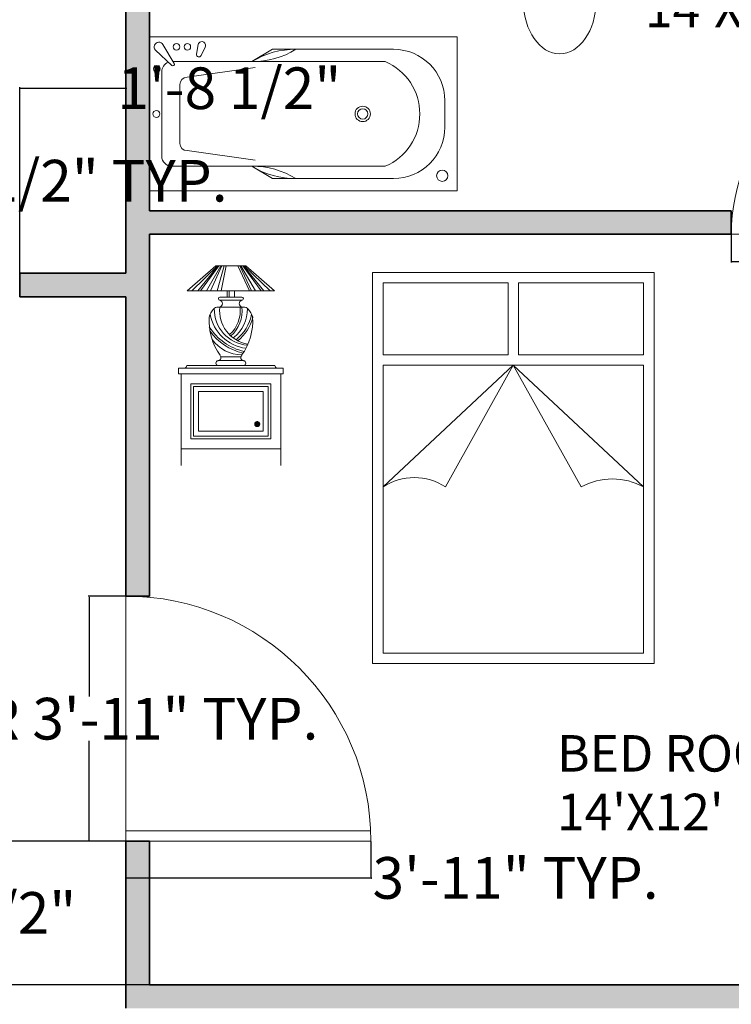
# Model space of a CAD drawing. Units: inches. Extents: x 638 to 1303, y 1 to 699.
# Tile 19 of 21: x 1026 to 1163, y 409 to 597. Entities that reach past the tile are written whole.
import ezdxf

# ---------------------------------------------------------------- set-up
doc = ezdxf.new("R2010")
doc.units = ezdxf.units.IN
doc.header["$MEASUREMENT"] = 0
for name, color, linetype, lineweight in [('A-ANNO-DIMS', 2, 'Continuous', 18), ('A-AREA-IDEN', 7, 'Continuous', 18), ('A-DOOR', 4, 'Continuous', 18), ('A-FLOR-FIXT', 9, 'Continuous', 18), ('A-WALL', 7, 'Continuous', 35), ('Furniture', 7, 'Continuous', 15)]:
    doc.layers.add(name, color=color, linetype=linetype, lineweight=lineweight)
doc.layers.add('A-WALL-PATT', color=143, linetype='Continuous', lineweight=13, true_color=0x7aafdf)
doc.styles.get("Standard").update_dxf_attribs({"font": 'arial.ttf'})
doc.dimstyles.get("Standard").update_dxf_attribs({"dimtxt": 8, "dimasz": 0.18, "dimexe": 0.18, "dimexo": 0.0625, "dimgap": 0.09, "dimtad": 0, "dimtih": 1, "dimtoh": 1, "dimdec": 4, "dimzin": 0, "dimdsep": 46, "dimlunit": 3, "dimtxsty": 'Standard', "dimcen": 0.09, "dimadec": 0, "dimazin": 0, "dimtfac": 1, "dimtdec": 4, "dimtofl": 0, "dimtmove": 0, "dimatfit": 3, "dimfxl": 1, "dimtolj": 1, "dimtzin": 0, "dimarcsym": 0})

# ---------------------------------------------------------------- blocks, each defined once
blk = doc.blocks.new('DOOR-SWING-47')
for p, q in [((45, 0), (45, 46.96)), ((47, 0), (47, 47)), ((0, 0), (47, 0))]:
    blk.add_line(p, q)
blk.add_arc((47, 0), 47, 90, 180)
blk = doc.blocks.new('DOOR-SWING-35')
for p, q in [((33, 0), (33, 34.94)), ((35, 0), (35, 35)), ((0, 0), (35, 0))]:
    blk.add_line(p, q)
blk.add_arc((35, 0), 35, 90, 180)
blk = doc.blocks.new('*X4')
at = {"color": 0}
for p, q in [((120.5, 200.05), (120.95, 200.5)), ((121, 199.5), (120.5, 200)), ((120.51, 199.89), (121.11, 200.49)), ((121.15, 199.52), (120.52, 200.15)), ((120.56, 199.76), (121.24, 200.44)), ((120.76, 199.56), (120.56, 199.76)), ((121.27, 199.58), (120.58, 200.27)), ((120.64, 199.66), (121.34, 200.36)), ((121.37, 199.66), (120.66, 200.37)), ((120.73, 199.58), (121.42, 200.27)), ((121.44, 199.76), (120.76, 200.44)), ((120.86, 199.52), (121.48, 200.14)), ((121.49, 199.89), (120.89, 200.49)), ((121.01, 199.5), (121.5, 199.99)), ((121.5, 200.06), (121.06, 200.5)), ((121.26, 199.57), (121.43, 199.74))]:
    blk.add_line(p, q, dxfattribs=at)
blk = doc.blocks.new('BEDSIDE-UNIT-WITH-LAMP')
for p, q in [((7.17, 38.27), (1.67, 33.48)), ((7.48, 38.27), (2.53, 33.48)), ((3.69, 33.48), (7.63, 38.27)), ((4.24, 33.48), (7.76, 38.27)), ((5.34, 33.48), (8.12, 38.27)), ((8.34, 38.27), (6.11, 33.48)), ((7.17, 38.27), (10.04, 38.27)), ((7.39, 33.48), (8.76, 38.27)), ((9.16, 38.27), (8.21, 33.48)), ((12.91, 38.27), (10.04, 38.27)), ((11.36, 38.27), (13.59, 33.48)), ((11.75, 38.27), (13.98, 33.48)), ((14.75, 33.48), (11.97, 38.27)), ((15.85, 33.48), (12.33, 38.27)), ((16.4, 33.48), (12.46, 38.27)), ((12.61, 38.27), (17.56, 33.48)), ((12.91, 38.27), (18.42, 33.48)), ((1.67, 33.48), (10.04, 33.48)), ((7.92, 32.29), (10.04, 32.29)), ((9.33, 32.29), (9.33, 33.48)), ((9.69, 32.29), (9.69, 33.48)), ((18.42, 33.48), (10.04, 33.48)), ((12.17, 32.29), (10.04, 32.29)), ((10.76, 32.29), (10.76, 33.48)), ((7.61, 30.38), (10.04, 30.38)), ((7.92, 31.69), (10.04, 31.69)), ((12.17, 31.69), (10.04, 31.69)), ((12.48, 30.38), (10.04, 30.38)), ((8.13, 20.83), (11.96, 20.83)), ((1.59, 19.13), (18.5, 19.13)), ((7.62, 20.09), (10.04, 20.09)), ((7.62, 19.13), (10.04, 19.13)), ((12.47, 20.09), (10.04, 20.09)), ((12.47, 19.13), (10.04, 19.13)), ((0, 18.66), (1.18, 18.66)), ((0, 18.66), (0, 17.54)), ((0, 17.54), (0.48, 17.54)), ((0.48, 17.54), (19.61, 17.54)), ((0.48, 17.54), (0.48, 0)), ((1.18, 18.66), (18.91, 18.66)), ((20.09, 18.66), (18.91, 18.66)), ((19.61, 17.54), (19.61, 0)), ((20.09, 17.54), (19.61, 17.54)), ((20.09, 18.66), (20.09, 17.54)), ((2.39, 15.63), (2.39, 5.1)), ((2.39, 15.63), (17.7, 15.63)), ((2.87, 15.15), (2.87, 5.58)), ((2.87, 15.15), (17.22, 15.15)), ((17.22, 15.15), (17.22, 5.58)), ((17.7, 15.63), (17.7, 5.1)), ((3.83, 14.19), (3.83, 6.54)), ((3.83, 14.19), (16.26, 14.19)), ((16.26, 14.19), (16.26, 6.54)), ((3.83, 6.54), (16.26, 6.54)), ((2.39, 5.1), (17.7, 5.1)), ((2.87, 5.58), (17.22, 5.58)), ((0.48, 3.19), (19.61, 3.19))]:
    blk.add_line(p, q)
blk.add_circle((15.11, 7.93), 0.478)
for centre, radius, start, end in [((7.95, 31.99), 0.301, 96.0644, 263.9356), ((12.14, 31.99), 0.301, 276.0644, 83.9356), ((7.61, 29.18), 1.2, 90, 137.4597), ((7.75, 31.04), 0.677, 281.8983, 74.8511), ((14.31, 29.63), 6.43, 173.3103, 261.113), ((5.78, 29.63), 6.07, 311.5876, 6.6897), ((5.78, 29.63), 6.43, 311.5876, 6.6897), ((12.34, 31.04), 0.677, 105.1489, 258.1017), ((12.48, 29.18), 1.2, 42.5403, 90), ((17.45, 27.82), 11.6, 176.8022, 215.2924), ((9.63, 27.32), 3.94, 137.4597, 163.1575), ((14, 30.46), 8.06, 190.3097, 262.4706), ((13.81, 29.96), 6.94, 178.6681, 265.1492), ((6.28, 29.96), 6.94, 307.422, 1.3319), ((6.09, 30.46), 8.06, 307.8159, 349.6903), ((6.09, 30.46), 8.42, 308.8588, 345.4877), ((2.64, 27.82), 11.6, 324.7076, 3.1978), ((10.46, 27.32), 3.94, 16.8425, 42.5403), ((14.79, 32.06), 10.42, 211.5602, 257.9287), ((14.79, 32.06), 10.78, 215.6196, 257.2465), ((12.31, 28.5), 7.31, 216.5807, 268.9053), ((7.53, 20.69), 0.609, 278.5359, 43.5342), ((12.56, 20.69), 0.609, 136.4658, 261.4641), ((1.05, 19.19), 0.546, 283.3604, 354.4124), ((7.65, 19.61), 0.479, 93.7182, 266.2818), ((12.44, 19.61), 0.479, 273.7182, 86.2818), ((19.04, 19.19), 0.546, 185.5876, 256.6396)]:
    blk.add_arc(centre, radius, start, end)
at = {"xscale": 0.956691, "yscale": 0.956691, "zscale": 0.956691}
blk.add_blockref('*X4', (-100.65, -183.4), dxfattribs=at)
blk = doc.blocks.new('*D26')
at = {"layer": 'A-ANNO-DIMS', "color": 0, "lineweight": -2, "transparency": 16777216}
for p, q in [((1046.68, 486.87), (1039.51, 486.87)), ((1039.69, 486.69), (1039.69, 467.61)), ((1039.69, 440.05), (1039.69, 459.14)), ((1046.68, 439.87), (1039.51, 439.87))]:
    blk.add_line(p, q, dxfattribs=at)
at = {"layer": 'A-ANNO-DIMS', "color": 0, "transparency": 16777216}
for points in [[(1039.66, 486.69), (1039.72, 486.69), (1039.69, 486.87)], [(1039.66, 440.05), (1039.72, 440.05), (1039.69, 439.87)]]:
    blk.add_solid(points, dxfattribs=at)
at = {"layer": 'Defpoints', "color": 0, "transparency": 16777216}
for p in [(1046.74, 486.87), (1039.69, 439.87), (1046.74, 439.87)]:
    blk.add_point(p, dxfattribs=at)
at = {"layer": 'A-ANNO-DIMS', "color": 0, "transparency": 16777216, "insert": (1039.69, 463.37), "char_height": 8, "attachment_point": 5}
blk.add_mtext('\\A1;DOOR 3\'-11" TYP.', dxfattribs=at)
blk = doc.blocks.new('*D27')
at = {"layer": 'A-ANNO-DIMS', "color": 0, "lineweight": -2, "transparency": 16777216}
for p, q in [((1046.74, 439.81), (1046.74, 432.64)), ((1093.74, 439.81), (1093.74, 432.64)), ((1046.92, 432.82), (1093.56, 432.82)), ((1093.74, 432.82), (1093.92, 432.82))]:
    blk.add_line(p, q, dxfattribs=at)
at = {"layer": 'A-ANNO-DIMS', "color": 0, "transparency": 16777216}
for points in [[(1046.92, 432.85), (1046.92, 432.79), (1046.74, 432.82)], [(1093.56, 432.85), (1093.56, 432.79), (1093.74, 432.82)]]:
    blk.add_solid(points, dxfattribs=at)
at = {"layer": 'Defpoints', "color": 0, "transparency": 16777216}
for p in [(1046.74, 439.87), (1093.74, 439.87), (1093.74, 432.82)]:
    blk.add_point(p, dxfattribs=at)
at = {"layer": 'A-ANNO-DIMS', "color": 0, "transparency": 16777216, "insert": (1121.5, 432.82), "char_height": 8, "attachment_point": 5}
blk.add_mtext('\\A1;3\'-11" TYP.', dxfattribs=at)
blk = doc.blocks.new('*D28')
at = {"layer": 'A-ANNO-DIMS', "color": 0, "lineweight": -2, "transparency": 16777216}
for p, q in [((1162.9, 556.26), (1162.9, 550.89)), ((1197.9, 556.26), (1197.9, 550.89)), ((1163.08, 551.07), (1197.72, 551.07)), ((1197.9, 551.07), (1198.08, 551.07))]:
    blk.add_line(p, q, dxfattribs=at)
at = {"layer": 'A-ANNO-DIMS', "color": 0, "transparency": 16777216}
for points in [[(1163.08, 551.1), (1163.08, 551.04), (1162.9, 551.07)], [(1197.72, 551.1), (1197.72, 551.04), (1197.9, 551.07)]]:
    blk.add_solid(points, dxfattribs=at)
at = {"layer": 'Defpoints', "color": 0, "transparency": 16777216}
for p in [(1162.9, 556.32), (1197.9, 556.32), (1197.9, 551.07)]:
    blk.add_point(p, dxfattribs=at)
at = {"layer": 'A-ANNO-DIMS', "color": 0, "transparency": 16777216, "insert": (1243.77, 551.07), "char_height": 8, "attachment_point": 5}
blk.add_mtext('\\A1;DOOR 2\'-11" TYP.', dxfattribs=at)
blk = doc.blocks.new('*D40')
at = {"layer": 'A-ANNO-DIMS', "color": 0, "lineweight": -2, "transparency": 16777216}
for p, q in [((974.2, 566.4), (974.84, 566.4)), ((974.66, 566.4), (974.66, 566.58)), ((974.66, 566.58), (974.84, 566.58)), ((974.66, 563.13), (974.66, 566.22)), ((974.2, 562.95), (974.84, 562.95))]:
    blk.add_line(p, q, dxfattribs=at)
at = {"layer": 'A-ANNO-DIMS', "color": 0, "transparency": 16777216}
for points in [[(974.63, 566.22), (974.69, 566.22), (974.66, 566.4)], [(974.63, 563.13), (974.69, 563.13), (974.66, 562.95)]]:
    blk.add_solid(points, dxfattribs=at)
at = {"layer": 'Defpoints', "color": 0, "transparency": 16777216}
for p in [(974.14, 566.4), (974.66, 566.4), (974.14, 562.95)]:
    blk.add_point(p, dxfattribs=at)
at = {"layer": 'A-ANNO-DIMS', "color": 0, "transparency": 16777216, "insert": (1021.15, 566.58), "char_height": 8, "attachment_point": 5}
blk.add_mtext('\\A1;TAP 0\'-3 1/2" TYP.', dxfattribs=at)
blk = doc.blocks.new('*D65')
at = {"layer": 'A-ANNO-DIMS', "color": 0, "lineweight": -2, "transparency": 16777216}
for p, q in [((1051.18, 439.87), (1015.56, 439.87)), ((1015.74, 439.69), (1015.74, 430.33)), ((1015.74, 412.5), (1015.74, 421.87)), ((1051.18, 412.32), (1015.56, 412.32))]:
    blk.add_line(p, q, dxfattribs=at)
at = {"layer": 'A-ANNO-DIMS', "color": 0, "transparency": 16777216}
for points in [[(1015.71, 439.69), (1015.77, 439.69), (1015.74, 439.87)], [(1015.71, 412.5), (1015.77, 412.5), (1015.74, 412.32)]]:
    blk.add_solid(points, dxfattribs=at)
at = {"layer": 'Defpoints', "color": 0, "transparency": 16777216}
for p in [(1015.74, 439.87), (1051.24, 439.87), (1051.24, 412.32)]:
    blk.add_point(p, dxfattribs=at)
at = {"layer": 'A-ANNO-DIMS', "color": 0, "transparency": 16777216, "insert": (1015.74, 426.1), "char_height": 8, "attachment_point": 5}
blk.add_mtext('\\A1;2\'-3 1/2"', dxfattribs=at)
blk = doc.blocks.new('*D67')
at = {"layer": 'A-ANNO-DIMS', "color": 0, "lineweight": -2, "transparency": 16777216}
for p, q in [((1026.36, 548.88), (1026.36, 584.5)), ((1026.54, 584.32), (1046.56, 584.32)), ((1046.74, 548.88), (1046.74, 584.5)), ((1046.74, 584.32), (1046.92, 584.32))]:
    blk.add_line(p, q, dxfattribs=at)
at = {"layer": 'A-ANNO-DIMS', "color": 0, "transparency": 16777216}
for points in [[(1026.54, 584.35), (1026.54, 584.29), (1026.36, 584.32)], [(1046.56, 584.35), (1046.56, 584.29), (1046.74, 584.32)]]:
    blk.add_solid(points, dxfattribs=at)
at = {"layer": 'Defpoints', "color": 0, "transparency": 16777216}
for p in [(1046.74, 584.32), (1026.36, 548.82), (1046.74, 548.82)]:
    blk.add_point(p, dxfattribs=at)
at = {"layer": 'A-ANNO-DIMS', "color": 0, "transparency": 16777216, "insert": (1066.59, 584.32), "char_height": 8, "attachment_point": 5}
blk.add_mtext('\\A1;1\'-8 1/2"', dxfattribs=at)

msp = doc.modelspace()

# ---------------------------------------------------------------- hatches: boundary and pattern name
at = {"layer": 'A-WALL-PATT'}
h = msp.add_hatch(color=256, dxfattribs=at)
h.dxf.hatch_style = 1
h.paths.add_polyline_path([(973.34524, 629.81895), (793.35541, 629.81895), (793.35541, 620.81895), (850.23798, 620.81895), (922.23798, 620.81895), (922.23798, 524.81895), (908.94335, 524.81895), (908.94335, 520.31895), (926.73798, 520.31895), (926.73798, 544.31895), (979.3571, 544.31895), (979.3571, 548.81895), (926.73798, 548.81895), (926.73798, 620.81895), (973.34524, 620.81895)])
h.paths.add_polyline_path([(758.35541, 629.81895), (697.23798, 629.81895), (697.23798, 586.77451), (706.23798, 586.77451), (706.23798, 620.81895), (758.35541, 620.81895)])
h.paths.add_polyline_path([(1075.85281, 629.81895), (1003.34524, 629.81895), (1003.34524, 620.81895), (1046.73798, 620.81895), (1046.73798, 560.81895), (1046.73798, 548.81895), (1026.3571, 548.81895), (1026.3571, 544.31895), (1046.73798, 544.31895), (1046.73798, 486.87457), (1051.23798, 486.87457), (1051.23798, 556.31895), (1162.89753, 556.31895), (1162.89753, 560.81895), (1051.23798, 560.81895), (1051.23798, 620.81895), (1075.85281, 620.81895)])
h.paths.add_polyline_path([(1228.23798, 629.81895), (1105.85281, 629.81895), (1105.85281, 620.81895), (1219.23798, 620.81895), (1219.23798, 560.81895), (1197.89753, 560.81895), (1197.89753, 556.31895), (1219.23798, 556.31895), (1219.23798, 498.80084), (1228.23798, 498.80084)])
h.paths.add_polyline_path([(1051.23798, 439.87457), (1046.73798, 439.87457), (1046.73798, 407.81895), (1219.23798, 407.81895), (1219.23798, 381.66175), (1228.23798, 381.66175), (1228.23798, 451.80084), (1219.23798, 451.80084), (1219.23798, 412.31895), (1051.23798, 412.31895)])
h.paths.add_polyline_path([(1228.23798, 346.66175), (1219.23798, 346.66175), (1219.23798, 335.81895), (1046.73798, 335.81895), (1046.73798, 273.56895), (1051.23798, 273.56895), (1051.23798, 331.31895), (1219.23798, 331.31895), (1219.23798, 308.99654), (1228.23798, 308.99654)])
h.paths.add_polyline_path([(1228.23798, 261.99654), (1219.23798, 261.99654), (1219.23798, 211.31895), (1051.23798, 211.31895), (1051.23798, 226.56895), (1046.73798, 226.56895), (1046.73798, 211.31895), (983.84714, 211.31895), (983.84714, 206.81895), (1219.23798, 206.81895), (1219.23798, 166.83987), (1228.23798, 166.83987)])
h.paths.add_polyline_path([(1228.23798, 119.83987), (1219.23798, 119.83987), (1219.23798, 50.81895), (1197.89277, 50.81895), (1197.89277, 41.81895), (1228.23798, 41.81895)])
h.paths.add_polyline_path([(1162.89277, 50.81895), (1069.02949, 50.81895), (1069.02949, 41.81895), (1162.89277, 41.81895)])
h.paths.add_polyline_path([(1010.02949, 50.81895), (941.89631, 50.81895), (917.77455, 50.81895), (917.77455, 41.81895), (941.89631, 41.81895), (1010.02949, 41.81895)])
h.paths.add_polyline_path([(882.77455, 50.81895), (854.73798, 50.81895), (854.73798, 145.50379), (850.23798, 145.50379), (850.23798, 50.81895), (793.49755, 50.81895), (793.49755, 41.81895), (882.77455, 41.81895)])
h.paths.add_polyline_path([(746.49755, 50.81895), (706.23798, 50.81895), (706.23798, 96.57416), (697.23798, 96.57416), (697.23798, 41.81895), (746.49755, 41.81895)])
h.paths.add_polyline_path([(706.23798, 206.81895), (714.01165, 206.81895), (714.01165, 211.31895), (706.23798, 211.31895), (706.23798, 251.21966), (697.23798, 251.21966), (697.23798, 143.57416), (706.23798, 143.57416)])
h.paths.add_polyline_path([(923.84714, 211.31895), (854.73798, 211.31895), (854.73798, 397.8313), (850.23798, 397.8313), (850.23798, 388.31895), (747.9539, 388.31895), (747.9539, 383.81895), (850.23798, 383.81895), (850.23798, 311.81895), (706.23798, 311.81895), (706.23798, 342.78787), (697.23798, 342.78787), (697.23798, 281.21966), (706.23798, 281.21966), (706.23798, 307.31895), (850.23798, 307.31895), (850.23798, 211.31895), (749.01165, 211.31895), (749.01165, 206.81895), (850.23798, 206.81895), (850.23798, 192.50379), (854.73798, 192.50379), (854.73798, 206.81895), (923.84714, 206.81895)])
h.paths.add_polyline_path([(706.23798, 434.70471), (697.23798, 434.70471), (697.23798, 372.78787), (706.23798, 372.78787), (706.23798, 383.81895), (712.9539, 383.81895), (712.9539, 388.31895), (706.23798, 388.31895)])
h.paths.add_polyline_path([(706.23798, 520.31895), (850.23798, 520.31895), (850.23798, 444.8313), (854.73798, 444.8313), (854.73798, 520.31895), (861.94335, 520.31895), (861.94335, 524.81895), (706.23798, 524.81895), (706.23798, 551.77451), (697.23798, 551.77451), (697.23798, 481.70471), (706.23798, 481.70471)])

# ---------------------------------------------------------------- linework, layer by layer
at = {"layer": 'A-FLOR-FIXT'}
for p, q in [((1110.29298, 594.15328), (1051.23798, 594.15328)), ((1051.23798, 594.15328), (1051.23798, 564.62578)), ((1110.29298, 564.62578), (1110.29298, 594.15328)), ((1052.38977, 591.6405), (1055.53451, 588.6848)), ((1056.01997, 589.07689), (1053.83167, 592.70751)), ((1060.58724, 592.70901), (1060.28128, 590.88136)), ((1061.17471, 590.6022), (1061.93761, 592.22346)), ((1070.92298, 589.42888), (1074.85998, 591.79108)), ((1098.08828, 591.79108), (1074.85998, 591.79108)), ((1096.51348, 589.42888), (1055.80781, 589.42888)), ((1058.46905, 586.41707), (1071.56509, 588.28012)), ((1053.60018, 587.46038), (1053.60018, 571.31868)), ((1057.0911, 585.03912), (1057.0911, 573.73993)), ((1107.93078, 576.83048), (1107.93078, 581.94858)), ((1058.46905, 572.36198), (1071.56509, 570.49893)), ((1055.56868, 569.35018), (1096.51348, 569.35018)), ((1070.92298, 569.35018), (1074.85998, 566.98798)), ((1074.85998, 566.98798), (1098.08828, 566.98798)), ((1051.23798, 564.62578), (1110.29298, 564.62578))]:
    msp.add_line(p, q, dxfattribs=at)
for centre, radius in [((1056.46336, 592.28321), 0.62765), ((1058.52895, 592.28321), 0.62765), ((1052.65833, 588.0383), 0.62765), ((1052.57971, 579.38953), 0.65561), ((1092.17082, 579.38953), 1.47637), ((1092.17082, 579.38953), 0.98425), ((1107.44261, 567.54094), 1.08553)]:
    msp.add_circle(centre, radius, dxfattribs=at)
for centre, radius, start, end in [((1053.04974, 592.25641), 0.90272, 29.9808131, 223.0225183), ((1061.29018, 592.54341), 0.72218, 333.702153, 166.7438582), ((1079.21809, 576.04997), 15.74179, 89.4650067, 121.7995067), ((1071.06996, 605.16998), 15.74179, 269.4650067, 301.7995067), ((1098.08828, 581.94858), 9.8425, 0, 90), ((1060.74723, 590.80336), 0.47244, 170.4962776, 334.8001843), ((1092.19591, 579.38953), 10.9284, 293.2708467, 66.7291533), ((1055.56868, 587.46038), 1.9685, 110.5848527, 180), ((1055.75022, 588.9143), 0.31496, 226.7749378, 31.0788444), ((1055.75022, 588.9143), 0.31496, 226.7749378, 31.0788444), ((1058.46905, 585.03912), 1.37795, 90, 180), ((1098.08828, 576.83048), 9.8425, 270, 0), ((1058.46905, 573.73993), 1.37795, 180, 270), ((1055.56868, 571.31868), 1.9685, 180, 270), ((1071.06996, 553.60907), 15.74179, 58.2004933, 90.5349933), ((1079.21809, 582.72908), 15.74179, 238.2004933, 270.5349933)]:
    msp.add_arc(centre, radius, start, end, dxfattribs=at)
msp.add_ellipse((1129.96915, 600.8465), major_axis=(0, -9.91352), ratio=0.7, dxfattribs=at)
at = {"layer": 'A-WALL'}
for p, q in [((1046.73798, 620.81895), (1046.73798, 560.81895)), ((1051.23798, 620.81895), (1051.23798, 560.81895)), ((1046.73798, 560.81895), (1046.73798, 548.81895)), ((1162.89753, 560.81895), (1051.23798, 560.81895)), ((1162.89753, 560.81895), (1162.89753, 556.31895)), ((1051.23798, 556.31895), (1051.23798, 486.87457)), ((1162.89753, 556.31895), (1051.23798, 556.31895)), ((1046.73798, 548.81895), (1026.3571, 548.81895)), ((1026.3571, 548.81895), (1026.3571, 544.31895)), ((1046.73798, 544.31895), (1026.3571, 544.31895)), ((1046.73798, 544.31895), (1046.73798, 486.87457)), ((1046.73798, 486.87457), (1051.23798, 486.87457)), ((1046.73798, 439.87457), (1051.23798, 439.87457)), ((1046.73798, 439.87457), (1046.73798, 407.81895)), ((1051.23798, 439.87457), (1051.23798, 412.31895)), ((1219.23798, 412.31895), (1051.23798, 412.31895))]:
    msp.add_line(p, q, dxfattribs=at)
at = {"layer": 'Furniture'}
for p, q in [((1148.07306, 548.95689), (1094.07306, 548.95689)), ((1094.07306, 548.95689), (1094.07306, 473.95689)), ((1148.07306, 473.95689), (1148.07306, 548.95689)), ((1096.07306, 546.95689), (1096.07306, 533.18775)), ((1120.07306, 546.95689), (1096.07306, 546.95689)), ((1120.07306, 533.18775), (1120.07306, 546.95689)), ((1146.07306, 546.95689), (1122.07306, 546.95689)), ((1122.07306, 533.18775), (1122.07306, 546.95689)), ((1146.07306, 533.18775), (1146.07306, 546.95689)), ((1096.07306, 533.18775), (1120.07306, 533.18775)), ((1122.07306, 533.18775), (1146.07306, 533.18775)), ((1096.07306, 531.18775), (1146.07306, 531.18775)), ((1096.07306, 531.18775), (1096.07306, 475.95689)), ((1121.07306, 531.18775), (1096.07306, 507.84562)), ((1108.07306, 507.84562), (1121.07306, 531.18775)), ((1121.07306, 531.18775), (1146.07306, 507.84562)), ((1134.07306, 507.84562), (1121.07306, 531.18775)), ((1146.07306, 475.95689), (1146.07306, 531.18775)), ((1096.07306, 475.95689), (1146.07306, 475.95689)), ((1094.07306, 473.95689), (1148.07306, 473.95689))]:
    msp.add_line(p, q, dxfattribs=at)
for centre, radius, start, end in [((1102.07306, 498.59448), 11.0265, 57.0338377, 122.9661623), ((1140.07306, 496.68671), 12.66971, 61.7336769, 118.2663231)]:
    msp.add_arc(centre, radius, start, end, dxfattribs=at)

# ---------------------------------------------------------------- block references
at = {"layer": 'A-DOOR'}
msp.add_blockref('DOOR-SWING-35', (1162.898, 556.319), dxfattribs=at)
at = {"layer": 'A-DOOR', "rotation": 270.0000000000002}
msp.add_blockref('DOOR-SWING-47', (1046.73803, 486.87492), dxfattribs=at)
at = {"layer": 'Furniture'}
msp.add_blockref('BEDSIDE-UNIT-WITH-LAMP', (1056.831, 511.968), dxfattribs=at)

# ---------------------------------------------------------------- texts
at = {"layer": 'A-AREA-IDEN'}
for s, p in [("14'X5'", (1146.35423, 596.02968)), ('BED ROOM', (1129.45331, 453.22006)), ("14'X12'", (1129.45331, 441.97518))]:
    msp.add_text(s, height=7, dxfattribs=at).set_placement(p)

# ---------------------------------------------------------------- dimensions: what is measured, and where the dimension line sits
at = {"layer": 'A-ANNO-DIMS'}
dim = msp.add_linear_dim(base=(1046.73798, 584.31895), p1=(1026.35711, 548.81895), p2=(1046.73798, 548.81895), dimstyle='Standard', override={"dimdec": 1, "dimlfac": 1, "dimrnd": 0, "dimzin": 1, "dimdsep": 46, "dimlunit": 4, "dimfrac": 2}, dxfattribs=at)
dim.commit()
dim.dimension.update_dxf_attribs({"geometry": '*D67', "text_midpoint": (1066.58506, 584.31895)})
for base, p1, p2, angle, text, picture, middle in [((974.65728, 566.40113), (974.14026, 562.95435), (974.14026, 566.40113), 90, 'TAP <> TYP.', '*D40', (1021.15102, 566.58113)), ((1039.68798, 439.87457), (1046.73798, 486.87457), (1046.73798, 439.87457), 270, 'DOOR <> TYP.', '*D26', (1039.68798, 463.37457)), ((1093.73798, 432.82457), (1046.73798, 439.87457), (1093.73798, 439.87457), 0, '<> TYP.', '*D27', (1121.49502, 432.82457))]:
    dim = msp.add_linear_dim(base=base, p1=p1, p2=p2, angle=angle, text=text, dimstyle='Standard', override={"dimdec": 1, "dimlfac": 1, "dimrnd": 0, "dimzin": 1, "dimdsep": 46, "dimlunit": 4, "dimfrac": 2}, dxfattribs=at)
    dim.commit()
    dim.dimension.update_dxf_attribs({"geometry": picture, "text_midpoint": middle})
dim = msp.add_linear_dim(base=(1197.89753, 551.06895), p1=(1162.89753, 556.31895), p2=(1197.89753, 556.31895), text='DOOR <> TYP.', dimstyle='Standard', override={"dimdec": 1, "dimlfac": 1, "dimrnd": 0, "dimzin": 1, "dimdsep": 46, "dimlunit": 4, "dimfrac": 2}, dxfattribs=at)
dim.commit()
dim.dimension.update_dxf_attribs({"geometry": '*D28', "text_midpoint": (1243.77462, 551.06895)})
dim = msp.add_linear_dim(base=(1015.73798, 439.87457), p1=(1051.23798, 412.31895), p2=(1051.23798, 439.87457), angle=90, dimstyle='Standard', override={"dimdec": 1, "dimlfac": 1, "dimrnd": 0, "dimzin": 1, "dimdsep": 46, "dimlunit": 4, "dimfrac": 2}, dxfattribs=at)
dim.commit()
dim.dimension.update_dxf_attribs({"geometry": '*D65', "text_midpoint": (1015.73798, 426.09676)})

doc.saveas('drawing.dxf')
